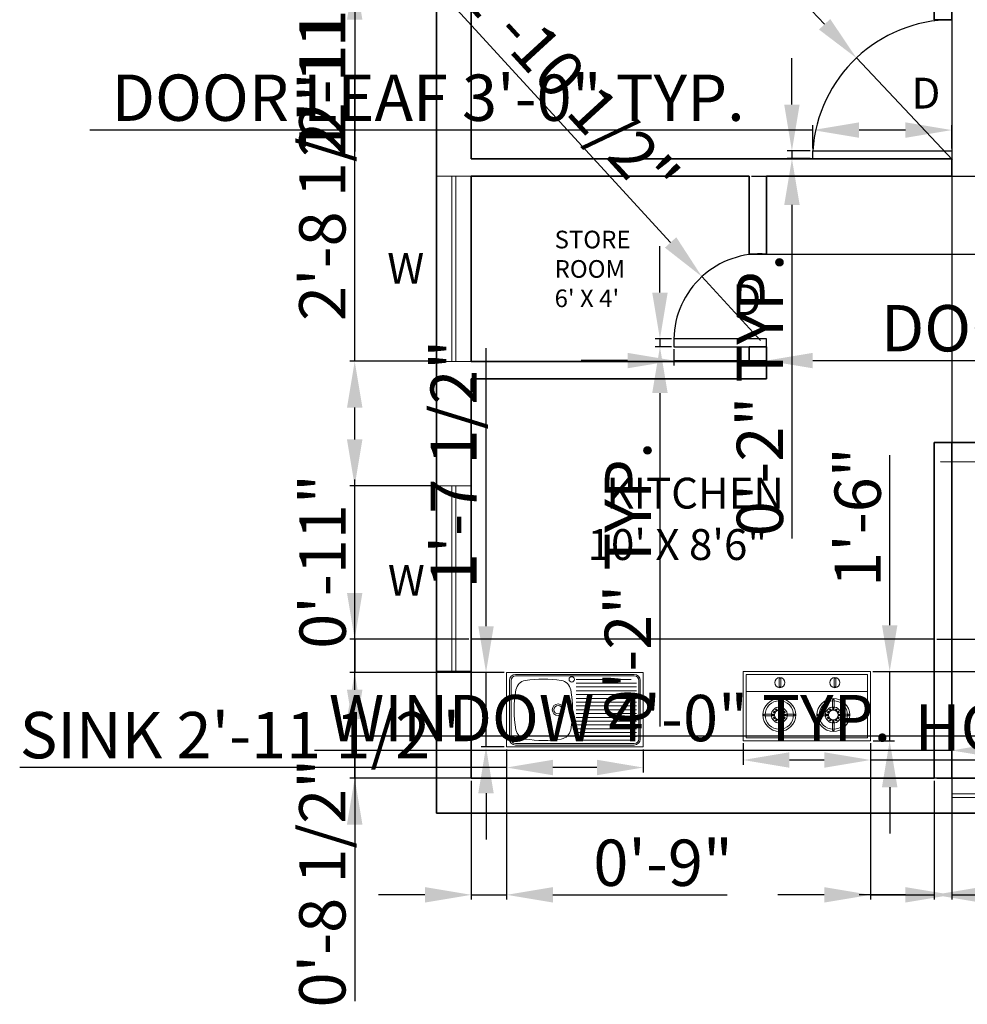
# Model space of a CAD drawing. Units: inches. Extents: x 2122 to 2726, y 1923 to 2370.
# Tile 1 of 6: x 2124 to 2370, y 1923 to 2178. Entities that reach past the tile are written whole.
import ezdxf

# ---------------------------------------------------------------- set-up
doc = ezdxf.new("R2010")
doc.units = ezdxf.units.IN
for name, color, linetype, lineweight in [('A-ANNO-DIMS', 2, 'Continuous', 18), ('A-ANNO-TEXT', 7, 'Continuous', 18), ('A-AREA-IDEN', 7, 'Continuous', 25), ('A-DOOR', 3, 'Continuous', 25), ('A-EQPM', 9, 'Continuous', 18), ('A-FLOR-CASE', 8, 'Continuous', 25), ('A-FLOR-FIXT', 9, 'Continuous', 18), ('A-GLAZ', 4, 'Continuous', 18), ('A-WALL', 7, 'Continuous', 35)]:
    doc.layers.add(name, color=color, linetype=linetype, lineweight=lineweight)
doc.styles.get("Standard").update_dxf_attribs({"font": 'arial.ttf'})
doc.dimstyles.new('ISO-25', dxfattribs={"dimtxt": 12, "dimasz": 12, "dimexe": 1.25, "dimexo": 0.625, "dimtad": 1, "dimlunit": 3, "dimtxsty": 'Standard', "dimcen": 2.5, "dimadec": 0, "dimazin": 0, "dimtfac": 1, "dimtmove": 0, "dimatfit": 3, "dimfxl": 1, "dimarcsym": 0})

# ---------------------------------------------------------------- blocks, each defined once
blk = doc.blocks.new('A$C06E242FC')
for p, q in [((0, 455.6), (0.5, 456.1)), ((0, 455.6), (0, 0.5)), ((838.9, 456.1), (0.5, 456.1)), ((838.9, 456.1), (839.4, 455.6)), ((839.4, 0.5), (839.4, 455.6)), ((20, 435.6), (20.5, 436.1)), ((20, 435.6), (20, 20.5)), ((818.9, 436.1), (20.5, 436.1)), ((237.3, 411.5), (237.3, 356.2)), ((248.9, 411.5), (237.3, 411.5)), ((248.9, 356.2), (248.9, 411.5)), ((599.3, 411.5), (610.9, 411.5)), ((599.3, 411.5), (599.3, 356.2)), ((610.9, 356.2), (610.9, 411.5)), ((819.4, 435.6), (818.9, 436.1)), ((819.4, 20.5), (819.4, 435.6)), ((20, 324.4), (819.4, 324.4)), ((237.3, 356.2), (248.9, 356.2)), ((599.3, 356.2), (610.9, 356.2)), ((232.7, 272.7), (232.7, 214)), ((244.9, 272.7), (232.7, 272.7)), ((244.9, 214), (244.9, 272.7)), ((588.1, 272.7), (588.1, 214)), ((600.3, 272.7), (588.1, 272.7)), ((600.3, 214), (600.3, 272.7)), ((232.7, 214), (244.9, 214)), ((588.1, 214), (600.3, 214)), ((136.3, 176), (136.3, 163.8)), ((194.9, 176), (136.3, 176)), ((136.3, 163.8), (194.9, 163.8)), ((194.9, 163.8), (194.9, 176)), ((282.9, 176.3), (282.9, 164.1)), ((341.6, 176.3), (282.9, 176.3)), ((282.9, 164.1), (341.6, 164.1)), ((341.6, 164.1), (341.6, 176.3)), ((550.3, 176), (491.7, 176)), ((491.7, 176), (491.7, 163.8)), ((491.7, 163.8), (550.3, 163.8)), ((550.3, 163.8), (550.3, 176)), ((638.3, 176.3), (638.3, 164.1)), ((697, 176.3), (638.3, 176.3)), ((638.3, 164.1), (697, 164.1)), ((697, 164.1), (697, 176.3)), ((245.2, 126.1), (233, 126.1)), ((233, 126.1), (233, 67.4)), ((233, 67.4), (245.2, 67.4)), ((245.2, 67.4), (245.2, 126.1)), ((600.6, 126.1), (588.3, 126.1)), ((588.3, 126.1), (588.3, 67.4)), ((588.3, 67.4), (600.6, 67.4)), ((600.6, 67.4), (600.6, 126.1)), ((0, 0.5), (0.5, 0)), ((20, 20.5), (20.5, 20)), ((20.5, 20), (818.9, 20)), ((818.9, 20), (819.4, 20.5)), ((838.9, 0), (839.4, 0.5)), ((0.5, 0), (838.9, 0))]:
    blk.add_line(p, q)
for centre, radius in [((242, 382.9), 33.3), ((604.1, 382.9), 33.3), ((238.9, 170.1), 108.3), ((238.9, 170.1), 93.3), ((594.3, 170.1), 108.3), ((594.3, 170.1), 93.3), ((238.9, 170.1), 52.6), ((238.9, 170.1), 32.6), ((219.5, 203.7), 4.84), ((238.9, 208.9), 4.84), ((258.4, 203.7), 4.84), ((594.3, 170.1), 52.6), ((594.3, 170.1), 32.6), ((574.9, 203.7), 4.84), ((594.3, 208.9), 4.84), ((613.7, 203.7), 4.84), ((200.1, 170.1), 4.84), ((205.3, 189.5), 4.84), ((205.3, 150.6), 4.84), ((219.5, 136.4), 4.84), ((238.9, 131.2), 4.84), ((258.4, 136.4), 4.84), ((272.6, 189.5), 4.84), ((272.6, 150.6), 4.84), ((277.8, 170.1), 4.84), ((555.5, 170.1), 4.84), ((560.7, 189.5), 4.84), ((560.7, 150.6), 4.84), ((574.9, 136.4), 4.84), ((594.3, 131.2), 4.84), ((613.7, 136.4), 4.84), ((628, 189.5), 4.84), ((628, 150.6), 4.84), ((633.2, 170.1), 4.84)]:
    blk.add_circle(centre, radius)
blk = doc.blocks.new('A$C0C3933DC')
for p, q in [((0, 490), (0, 0)), ((900, 490), (0, 490)), ((59.5, 477.5), (450, 477.5)), ((59.5, 467.5), (450, 467.5)), ((840.5, 477.5), (450, 477.5)), ((840.5, 467.5), (450, 467.5)), ((900, 0), (900, 490)), ((19.5, 52.5), (19.5, 437.5)), ((29.5, 52.5), (29.5, 437.5)), ((441, 420), (45, 420)), ((441, 395), (45, 395)), ((441, 445), (80.7, 445)), ((870.5, 52.5), (870.5, 437.5)), ((880.5, 52.5), (880.5, 437.5)), ((441, 370), (45, 370)), ((441, 345), (45, 345)), ((441, 320), (45, 320)), ((441, 295), (45, 295)), ((441, 270), (45, 270)), ((441, 245), (45, 245)), ((441, 220), (45, 220)), ((441, 195), (45, 195)), ((441, 170), (45, 170)), ((441, 145), (45, 145)), ((441, 120), (45, 120)), ((441, 95), (45, 95)), ((441, 70), (45, 70)), ((0, 0), (900, 0)), ((450, 22.5), (59.5, 22.5)), ((450, 12.5), (59.5, 12.5)), ((441, 45), (80.7, 45)), ((450, 22.5), (840.5, 22.5)), ((450, 12.5), (840.5, 12.5))]:
    blk.add_line(p, q)
for centre, radius in [((471, 445), 17.5), ((561, 245), 38), ((561, 245), 27.5)]:
    blk.add_circle(centre, radius)
for centre, radius, start, end in [((59.5, 437.5), 40, 90, 180), ((59.5, 437.5), 30, 90, 180), ((840.5, 437.5), 40, 0, 90), ((840.5, 437.5), 30, 0, 90), ((551.5, 363.5), 75, 99.07872, 169.88522), ((658, -303), 750, 80.92128, 99.07872), ((764.5, 363.5), 75, 10.11478, 80.92128), ((1216, 245), 750, 169.88522, 190.11478), ((100, 245), 750, 349.88522, 10.11478), ((551.5, 126.5), 75, 190.11478, 260.92128), ((764.5, 126.5), 75, 279.07872, 349.88522), ((59.5, 52.5), 40, 180, 270), ((59.5, 52.5), 30, 180, 270), ((658, 793), 750, 260.92128, 279.07872), ((840.5, 52.5), 30, 270, 0), ((840.5, 52.5), 40, 270, 0)]:
    blk.add_arc(centre, radius, start, end)
blk = doc.blocks.new('WIN-48IN')
for p, q in [((9, 48), (0, 48)), ((4, 0), (4, 48)), ((5, 0), (5, 48)), ((9, 0), (0, 0))]:
    blk.add_line(p, q)
blk = doc.blocks.new('DOOR-LEAF-36IN')
for p, q in [((0, 2), (36, 2)), ((0, 0), (0, 2)), ((36, 0), (0, 0)), ((36, 2), (36, 0))]:
    blk.add_line(p, q)
blk = doc.blocks.new('DOOR-LEAF-24IN')
for p, q in [((2, 24), (0, 24)), ((0, 24), (0, 0)), ((2, 0), (2, 24)), ((0, 0), (2, 0))]:
    blk.add_line(p, q)
blk = doc.blocks.new('*D18')
at = {"layer": 'A-ANNO-DIMS', "color": 0, "lineweight": -2, "transparency": 16777216}
for p, q in [((2366.01, 1982.36), (2366.01, 1990.19)), ((2414.01, 1982.36), (2414.01, 1990.19)), ((2366.01, 1988.94), (2200.91, 1988.94)), ((2402.01, 1988.94), (2378.01, 1988.94))]:
    blk.add_line(p, q, dxfattribs=at)
at = {"layer": 'A-ANNO-DIMS', "color": 0, "transparency": 16777216}
for points in [[(2378.01, 1990.94), (2378.01, 1986.94), (2366.01, 1988.94)], [(2402.01, 1990.94), (2402.01, 1986.94), (2414.01, 1988.94)]]:
    blk.add_solid(points, dxfattribs=at)
at = {"layer": 'Defpoints', "color": 0, "transparency": 16777216}
for p in [(2366.01, 1988.94), (2366.01, 1981.74), (2414.01, 1981.74)]:
    blk.add_point(p, dxfattribs=at)
at = {"layer": 'A-ANNO-DIMS', "color": 0, "transparency": 16777216, "insert": (2277.46, 1995.77), "char_height": 12, "attachment_point": 5}
blk.add_mtext('WINDOW 4\'-0" TYP.', dxfattribs=at)
blk = doc.blocks.new('*D22')
at = {"layer": 'A-ANNO-DIMS', "color": 0, "lineweight": -2, "transparency": 16777216}
for p, q in [((2330.01, 2144.86), (2330.01, 2150.89)), ((2366.01, 2144.86), (2366.01, 2150.89)), ((2330.01, 2149.64), (2142.68, 2149.64)), ((2354.01, 2149.64), (2342.01, 2149.64))]:
    blk.add_line(p, q, dxfattribs=at)
at = {"layer": 'A-ANNO-DIMS', "color": 0, "transparency": 16777216}
for points in [[(2342.01, 2151.64), (2342.01, 2147.64), (2330.01, 2149.64)], [(2354.01, 2151.64), (2354.01, 2147.64), (2366.01, 2149.64)]]:
    blk.add_solid(points, dxfattribs=at)
at = {"layer": 'Defpoints', "color": 0, "transparency": 16777216}
for p in [(2330.01, 2149.64), (2330.01, 2144.24), (2366.01, 2144.24)]:
    blk.add_point(p, dxfattribs=at)
at = {"layer": 'A-ANNO-DIMS', "color": 0, "transparency": 16777216, "insert": (2230.34, 2156.47), "char_height": 12, "attachment_point": 5}
blk.add_mtext('DOOR LEAF 3\'-0" TYP.', dxfattribs=at)
blk = doc.blocks.new('*D23')
at = {"layer": 'A-ANNO-DIMS', "color": 0, "lineweight": -2, "transparency": 16777216}
for p, q in [((2324.61, 2156.24), (2324.61, 2168.24)), ((2329.38, 2144.24), (2323.36, 2144.24)), ((2324.61, 2144.24), (2324.61, 2142.24)), ((2329.38, 2142.24), (2323.36, 2142.24)), ((2324.61, 2130.24), (2324.61, 2043.84))]:
    blk.add_line(p, q, dxfattribs=at)
at = {"layer": 'A-ANNO-DIMS', "color": 0, "transparency": 16777216}
for points in [[(2322.61, 2156.24), (2326.61, 2156.24), (2324.61, 2144.24)], [(2322.61, 2130.24), (2326.61, 2130.24), (2324.61, 2142.24)]]:
    blk.add_solid(points, dxfattribs=at)
at = {"layer": 'Defpoints', "color": 0, "transparency": 16777216}
for p in [(2330.01, 2144.24), (2324.61, 2142.24), (2330.01, 2142.24)]:
    blk.add_point(p, dxfattribs=at)
at = {"layer": 'A-ANNO-DIMS', "color": 0, "transparency": 16777216, "insert": (2317.86, 2081.04), "char_height": 12, "attachment_point": 5, "rotation": 90}
blk.add_mtext('0\'-2" TYP.', dxfattribs=at)
blk = doc.blocks.new('*D24')
at = {"layer": 'A-ANNO-DIMS', "color": 0, "lineweight": -2, "transparency": 16777216}
for p, q in [((2294.01, 2092.91), (2294.01, 2088.68)), ((2318.01, 2092.91), (2318.01, 2088.68)), ((2282.01, 2089.93), (2270.01, 2089.93)), ((2294.01, 2089.93), (2318.01, 2089.93)), ((2330.01, 2089.93), (2517.34, 2089.93))]:
    blk.add_line(p, q, dxfattribs=at)
at = {"layer": 'A-ANNO-DIMS', "color": 0, "transparency": 16777216}
for points in [[(2282.01, 2091.93), (2282.01, 2087.93), (2294.01, 2089.93)], [(2330.01, 2091.93), (2330.01, 2087.93), (2318.01, 2089.93)]]:
    blk.add_solid(points, dxfattribs=at)
at = {"layer": 'Defpoints', "color": 0, "transparency": 16777216}
for p in [(2294.01, 2093.53), (2318.01, 2093.53), (2318.01, 2089.93)]:
    blk.add_point(p, dxfattribs=at)
at = {"layer": 'A-ANNO-DIMS', "color": 0, "transparency": 16777216, "insert": (2429.67, 2096.76), "char_height": 12, "attachment_point": 5}
blk.add_mtext('DOOR LEAF 2\'-0" TYP.', dxfattribs=at)
blk = doc.blocks.new('*D25')
at = {"layer": 'A-ANNO-DIMS', "color": 0, "lineweight": -2, "transparency": 16777216}
for p, q in [((2290.41, 2107.53), (2290.41, 2119.53)), ((2293.38, 2095.53), (2289.16, 2095.53)), ((2290.41, 2095.53), (2290.41, 2093.53)), ((2293.38, 2093.53), (2289.16, 2093.53)), ((2290.41, 2081.53), (2290.41, 1995.13))]:
    blk.add_line(p, q, dxfattribs=at)
at = {"layer": 'A-ANNO-DIMS', "color": 0, "transparency": 16777216}
for points in [[(2288.41, 2107.53), (2292.41, 2107.53), (2290.41, 2095.53)], [(2288.41, 2081.53), (2292.41, 2081.53), (2290.41, 2093.53)]]:
    blk.add_solid(points, dxfattribs=at)
at = {"layer": 'Defpoints', "color": 0, "transparency": 16777216}
for p in [(2294.01, 2095.53), (2290.41, 2093.53), (2294.01, 2093.53)]:
    blk.add_point(p, dxfattribs=at)
at = {"layer": 'A-ANNO-DIMS', "color": 0, "transparency": 16777216, "insert": (2283.66, 2032.33), "char_height": 12, "attachment_point": 5, "rotation": 90}
blk.add_mtext('0\'-2" TYP.', dxfattribs=at)
blk = doc.blocks.new('*D30')
at = {"layer": 'A-ANNO-DIMS', "color": 0, "lineweight": -2, "transparency": 16777216}
for p, q in [((2311.94, 1990.8), (2311.94, 1985.22)), ((2344.99, 1990.8), (2344.99, 1985.22)), ((2323.94, 1986.47), (2332.99, 1986.47)), ((2344.99, 1986.47), (2430.48, 1986.47))]:
    blk.add_line(p, q, dxfattribs=at)
at = {"layer": 'A-ANNO-DIMS', "color": 0, "transparency": 16777216}
for points in [[(2323.94, 1988.47), (2323.94, 1984.47), (2311.94, 1986.47)], [(2332.99, 1988.47), (2332.99, 1984.47), (2344.99, 1986.47)]]:
    blk.add_solid(points, dxfattribs=at)
at = {"layer": 'Defpoints', "color": 0, "transparency": 16777216}
for p in [(2311.94, 1991.43), (2344.99, 1991.43), (2344.99, 1986.47)]:
    blk.add_point(p, dxfattribs=at)
at = {"layer": 'A-ANNO-DIMS', "color": 0, "transparency": 16777216, "insert": (2393.73, 1993.3), "char_height": 12, "attachment_point": 5}
blk.add_mtext('HOB 2\'-9"', dxfattribs=at)
blk = doc.blocks.new('*D31')
at = {"layer": 'A-ANNO-DIMS', "color": 0, "lineweight": -2, "transparency": 16777216}
for p, q in [((2349.95, 2021.39), (2349.95, 2065.4)), ((2345.62, 2009.39), (2351.2, 2009.39)), ((2349.95, 1991.43), (2349.95, 2009.39)), ((2345.62, 1991.43), (2351.2, 1991.43)), ((2349.95, 1979.43), (2349.95, 1967.43))]:
    blk.add_line(p, q, dxfattribs=at)
at = {"layer": 'A-ANNO-DIMS', "color": 0, "transparency": 16777216}
for points in [[(2347.95, 2021.39), (2351.95, 2021.39), (2349.95, 2009.39)], [(2347.95, 1979.43), (2351.95, 1979.43), (2349.95, 1991.43)]]:
    blk.add_solid(points, dxfattribs=at)
at = {"layer": 'Defpoints', "color": 0, "transparency": 16777216}
for p in [(2344.99, 2009.39), (2349.95, 2009.39), (2344.99, 1991.43)]:
    blk.add_point(p, dxfattribs=at)
at = {"layer": 'A-ANNO-DIMS', "color": 0, "transparency": 16777216, "insert": (2343.2, 2049.39), "char_height": 12, "attachment_point": 5, "rotation": 90}
blk.add_mtext('1\'-6"', dxfattribs=at)
blk = doc.blocks.new('*D32')
at = {"layer": 'A-ANNO-DIMS', "color": 0, "lineweight": -2, "transparency": 16777216}
for p, q in [((2250.66, 1989.21), (2250.66, 1983.27)), ((2286.09, 1989.21), (2286.09, 1983.27)), ((2250.66, 1984.52), (2124.5, 1984.52)), ((2274.09, 1984.52), (2262.66, 1984.52))]:
    blk.add_line(p, q, dxfattribs=at)
at = {"layer": 'A-ANNO-DIMS', "color": 0, "transparency": 16777216}
for points in [[(2262.66, 1986.52), (2262.66, 1982.52), (2250.66, 1984.52)], [(2274.09, 1986.52), (2274.09, 1982.52), (2286.09, 1984.52)]]:
    blk.add_solid(points, dxfattribs=at)
at = {"layer": 'Defpoints', "color": 0, "transparency": 16777216}
for p in [(2250.66, 1989.84), (2286.09, 1989.84), (2250.66, 1984.52)]:
    blk.add_point(p, dxfattribs=at)
at = {"layer": 'A-ANNO-DIMS', "color": 0, "transparency": 16777216, "insert": (2181.58, 1991.35), "char_height": 12, "attachment_point": 5}
blk.add_mtext('SINK 2\'-11 1/2"', dxfattribs=at)
blk = doc.blocks.new('*D33')
at = {"layer": 'A-ANNO-DIMS', "color": 0, "lineweight": -2, "transparency": 16777216}
for p, q in [((2245.34, 2021.13), (2245.34, 2093.11)), ((2250.03, 2009.13), (2244.09, 2009.13)), ((2245.34, 1989.84), (2245.34, 2009.13)), ((2250.03, 1989.84), (2244.09, 1989.84)), ((2245.34, 1977.84), (2245.34, 1965.84))]:
    blk.add_line(p, q, dxfattribs=at)
at = {"layer": 'A-ANNO-DIMS', "color": 0, "transparency": 16777216}
for points in [[(2243.34, 2021.13), (2247.34, 2021.13), (2245.34, 2009.13)], [(2243.34, 1977.84), (2247.34, 1977.84), (2245.34, 1989.84)]]:
    blk.add_solid(points, dxfattribs=at)
at = {"layer": 'Defpoints', "color": 0, "transparency": 16777216}
for p in [(2245.34, 2009.13), (2250.66, 2009.13), (2250.66, 1989.84)]:
    blk.add_point(p, dxfattribs=at)
at = {"layer": 'A-ANNO-DIMS', "color": 0, "transparency": 16777216, "insert": (2238.51, 2063.12), "char_height": 12, "attachment_point": 5, "rotation": 90}
blk.add_mtext('1\'-7 1/2"', dxfattribs=at)
blk = doc.blocks.new('*D40')
at = {"layer": 'A-ANNO-DIMS', "color": 0, "lineweight": -2, "transparency": 16777216}
for p, q in [((2362.13, 2017.74), (2622.46, 2017.74)), ((2621.21, 1993.74), (2621.21, 2005.74)), ((2362.13, 1981.74), (2622.46, 1981.74))]:
    blk.add_line(p, q, dxfattribs=at)
at = {"layer": 'A-ANNO-DIMS', "color": 0, "transparency": 16777216}
for points in [[(2619.21, 2005.74), (2623.21, 2005.74), (2621.21, 2017.74)], [(2619.21, 1993.74), (2623.21, 1993.74), (2621.21, 1981.74)]]:
    blk.add_solid(points, dxfattribs=at)
at = {"layer": 'Defpoints', "color": 0, "transparency": 16777216}
for p in [(2361.51, 2017.74), (2621.21, 2017.74), (2361.51, 1981.74)]:
    blk.add_point(p, dxfattribs=at)
at = {"layer": 'A-ANNO-DIMS', "color": 0, "transparency": 16777216, "insert": (2614.45, 1999.74), "char_height": 12, "attachment_point": 5, "rotation": 90}
blk.add_mtext('3\'-0"', dxfattribs=at)
blk = doc.blocks.new('*D45')
at = {"layer": 'A-ANNO-DIMS', "color": 0, "lineweight": -2, "transparency": 16777216}
for p, q in [((2211.31, 2089.74), (2211.31, 2163.05)), ((2231.88, 2089.74), (2210.06, 2089.74)), ((2211.31, 2069.49), (2211.31, 2077.74)), ((2231.88, 2057.49), (2210.06, 2057.49))]:
    blk.add_line(p, q, dxfattribs=at)
at = {"layer": 'A-ANNO-DIMS', "color": 0, "transparency": 16777216}
for points in [[(2209.31, 2077.74), (2213.31, 2077.74), (2211.31, 2089.74)], [(2209.31, 2069.49), (2213.31, 2069.49), (2211.31, 2057.49)]]:
    blk.add_solid(points, dxfattribs=at)
at = {"layer": 'Defpoints', "color": 0, "transparency": 16777216}
for p in [(2211.31, 2089.74), (2232.51, 2089.74), (2232.51, 2057.49)]:
    blk.add_point(p, dxfattribs=at)
at = {"layer": 'A-ANNO-DIMS', "color": 0, "transparency": 16777216, "insert": (2204.48, 2132.39), "char_height": 12, "attachment_point": 5, "rotation": 90}
blk.add_mtext('2\'-8 1/2"', dxfattribs=at)
blk = doc.blocks.new('*D50')
at = {"layer": 'A-ANNO-DIMS', "color": 0, "lineweight": -2, "transparency": 16777216}
for p, q in [((2366.01, 2189.61), (2366.01, 1950.29)), ((2385.88, 2189.61), (2385.88, 1950.29)), ((2354.01, 1951.54), (2342.01, 1951.54)), ((2366.01, 1951.54), (2385.88, 1951.54)), ((2397.88, 1951.54), (2441.9, 1951.54))]:
    blk.add_line(p, q, dxfattribs=at)
at = {"layer": 'A-ANNO-DIMS', "color": 0, "transparency": 16777216}
for points in [[(2354.01, 1953.54), (2354.01, 1949.54), (2366.01, 1951.54)], [(2397.88, 1953.54), (2397.88, 1949.54), (2385.88, 1951.54)]]:
    blk.add_solid(points, dxfattribs=at)
at = {"layer": 'Defpoints', "color": 0, "transparency": 16777216}
for p in [(2366.01, 2190.24), (2385.88, 2190.24), (2385.88, 1951.54)]:
    blk.add_point(p, dxfattribs=at)
at = {"layer": 'A-ANNO-DIMS', "color": 0, "transparency": 16777216, "insert": (2425.89, 1958.29), "char_height": 12, "attachment_point": 5}
blk.add_mtext('1\'-8"', dxfattribs=at)
blk = doc.blocks.new('*D51')
at = {"layer": 'A-ANNO-DIMS', "color": 0, "lineweight": -2, "transparency": 16777216}
for p, q in [((2211.31, 2209.57), (2211.31, 2282.68)), ((2465.88, 2197.57), (2210.06, 2197.57)), ((2211.31, 2190.24), (2211.31, 2197.57)), ((2465.88, 2190.24), (2210.06, 2190.24)), ((2211.31, 2178.24), (2211.31, 2166.24))]:
    blk.add_line(p, q, dxfattribs=at)
at = {"layer": 'A-ANNO-DIMS', "color": 0, "transparency": 16777216}
for points in [[(2209.31, 2209.57), (2213.31, 2209.57), (2211.31, 2197.57)], [(2209.31, 2178.24), (2213.31, 2178.24), (2211.31, 2190.24)]]:
    blk.add_solid(points, dxfattribs=at)
at = {"layer": 'Defpoints', "color": 0, "transparency": 16777216}
for p in [(2211.31, 2197.57), (2466.51, 2197.57), (2466.51, 2190.24)]:
    blk.add_point(p, dxfattribs=at)
at = {"layer": 'A-ANNO-DIMS', "color": 0, "transparency": 16777216, "insert": (2204.48, 2252.12), "char_height": 12, "attachment_point": 5, "rotation": 90}
blk.add_mtext('0\'-7 1/2"', dxfattribs=at)
blk = doc.blocks.new('*D52')
at = {"layer": 'A-ANNO-DIMS', "color": 0, "lineweight": -2, "transparency": 16777216}
for p, q in [((2621.21, 2149.74), (2621.21, 2161.74)), ((2314.13, 2137.74), (2622.46, 2137.74)), ((2621.21, 2137.74), (2621.21, 2117.53)), ((2314.13, 2117.53), (2622.46, 2117.53)), ((2621.21, 2105.53), (2621.21, 2061.51))]:
    blk.add_line(p, q, dxfattribs=at)
at = {"layer": 'A-ANNO-DIMS', "color": 0, "transparency": 16777216}
for points in [[(2619.21, 2149.74), (2623.21, 2149.74), (2621.21, 2137.74)], [(2619.21, 2105.53), (2623.21, 2105.53), (2621.21, 2117.53)]]:
    blk.add_solid(points, dxfattribs=at)
at = {"layer": 'Defpoints', "color": 0, "transparency": 16777216}
for p in [(2313.51, 2137.74), (2313.51, 2117.53), (2621.21, 2117.53)]:
    blk.add_point(p, dxfattribs=at)
at = {"layer": 'A-ANNO-DIMS', "color": 0, "transparency": 16777216, "insert": (2614.46, 2077.52), "char_height": 12, "attachment_point": 5, "rotation": 90}
blk.add_mtext('1\'-8"', dxfattribs=at)
blk = doc.blocks.new('*D53')
at = {"layer": 'A-ANNO-DIMS', "color": 0, "lineweight": -2, "transparency": 16777216}
for p, q in [((2250.66, 1989.21), (2250.66, 1950.29)), ((2241.51, 1981.11), (2241.51, 1950.29)), ((2229.51, 1951.54), (2217.51, 1951.54)), ((2241.51, 1951.54), (2250.66, 1951.54)), ((2262.66, 1951.54), (2307.81, 1951.54))]:
    blk.add_line(p, q, dxfattribs=at)
at = {"layer": 'A-ANNO-DIMS', "color": 0, "transparency": 16777216}
for points in [[(2229.51, 1953.54), (2229.51, 1949.54), (2241.51, 1951.54)], [(2262.66, 1953.54), (2262.66, 1949.54), (2250.66, 1951.54)]]:
    blk.add_solid(points, dxfattribs=at)
at = {"layer": 'Defpoints', "color": 0, "transparency": 16777216}
for p in [(2250.66, 1989.84), (2241.51, 1981.74), (2250.66, 1951.54)]:
    blk.add_point(p, dxfattribs=at)
at = {"layer": 'A-ANNO-DIMS', "color": 0, "transparency": 16777216, "insert": (2291.23, 1958.29), "char_height": 12, "attachment_point": 5}
blk.add_mtext('0\'-9"', dxfattribs=at)
blk = doc.blocks.new('*D54')
at = {"layer": 'A-ANNO-DIMS', "color": 0, "lineweight": -2, "transparency": 16777216}
for p, q in [((2211.31, 2029.74), (2211.31, 2041.74)), ((2240.88, 2017.74), (2210.06, 2017.74)), ((2211.31, 2017.74), (2211.31, 2009.13)), ((2250.03, 2009.13), (2210.06, 2009.13)), ((2211.31, 1997.13), (2211.31, 1924.02))]:
    blk.add_line(p, q, dxfattribs=at)
at = {"layer": 'A-ANNO-DIMS', "color": 0, "transparency": 16777216}
for points in [[(2209.31, 2029.74), (2213.31, 2029.74), (2211.31, 2017.74)], [(2209.31, 1997.13), (2213.31, 1997.13), (2211.31, 2009.13)]]:
    blk.add_solid(points, dxfattribs=at)
at = {"layer": 'Defpoints', "color": 0, "transparency": 16777216}
for p in [(2241.51, 2017.74), (2211.31, 2009.13), (2250.66, 2009.13)]:
    blk.add_point(p, dxfattribs=at)
at = {"layer": 'A-ANNO-DIMS', "color": 0, "transparency": 16777216, "insert": (2204.48, 1954.57), "char_height": 12, "attachment_point": 5, "rotation": 90}
blk.add_mtext('0\'-8 1/2"', dxfattribs=at)
blk = doc.blocks.new('*D55')
at = {"layer": 'A-ANNO-DIMS', "color": 0, "lineweight": -2, "transparency": 16777216}
for p, q in [((2344.97, 1990.8), (2344.97, 1950.29)), ((2361.51, 1981.11), (2361.51, 1950.29)), ((2332.97, 1951.54), (2320.97, 1951.54)), ((2344.97, 1951.54), (2361.51, 1951.54)), ((2373.51, 1951.54), (2445.49, 1951.54))]:
    blk.add_line(p, q, dxfattribs=at)
at = {"layer": 'A-ANNO-DIMS', "color": 0, "transparency": 16777216}
for points in [[(2332.97, 1953.54), (2332.97, 1949.54), (2344.97, 1951.54)], [(2373.51, 1953.54), (2373.51, 1949.54), (2361.51, 1951.54)]]:
    blk.add_solid(points, dxfattribs=at)
at = {"layer": 'Defpoints', "color": 0, "transparency": 16777216}
for p in [(2344.97, 1991.43), (2361.51, 1981.74), (2361.51, 1951.54)]:
    blk.add_point(p, dxfattribs=at)
at = {"layer": 'A-ANNO-DIMS', "color": 0, "transparency": 16777216, "insert": (2415.5, 1958.37), "char_height": 12, "attachment_point": 5}
blk.add_mtext('1\'-4 1/2"', dxfattribs=at)
blk = doc.blocks.new('*D56')
at = {"layer": 'A-ANNO-DIMS', "color": 0, "lineweight": -2, "transparency": 16777216}
for p, q in [((2621.21, 2029.74), (2621.21, 2102.85)), ((2362.13, 2017.74), (2622.46, 2017.74)), ((2621.21, 2009.39), (2621.21, 2017.74)), ((2345.6, 2009.39), (2622.46, 2009.39)), ((2621.21, 1997.39), (2621.21, 1985.39))]:
    blk.add_line(p, q, dxfattribs=at)
at = {"layer": 'A-ANNO-DIMS', "color": 0, "transparency": 16777216}
for points in [[(2619.21, 2029.74), (2623.21, 2029.74), (2621.21, 2017.74)], [(2619.21, 1997.39), (2623.21, 1997.39), (2621.21, 2009.39)]]:
    blk.add_solid(points, dxfattribs=at)
at = {"layer": 'Defpoints', "color": 0, "transparency": 16777216}
for p in [(2361.51, 2017.74), (2621.21, 2017.74), (2344.97, 2009.39)]:
    blk.add_point(p, dxfattribs=at)
at = {"layer": 'A-ANNO-DIMS', "color": 0, "transparency": 16777216, "insert": (2614.38, 2072.29), "char_height": 12, "attachment_point": 5, "rotation": 90}
blk.add_mtext('0\'-8 1/2"', dxfattribs=at)
blk = doc.blocks.new('*D59')
at = {"layer": 'A-ANNO-DIMS', "color": 0, "lineweight": -2, "transparency": 16777216}
for p, q in [((2211.31, 2004.66), (2211.31, 2059.13)), ((2481.63, 1992.66), (2210.06, 1992.66)), ((2211.31, 1981.74), (2211.31, 1992.66)), ((2470.38, 1981.74), (2210.06, 1981.74)), ((2211.31, 1969.74), (2211.31, 1957.74))]:
    blk.add_line(p, q, dxfattribs=at)
at = {"layer": 'A-ANNO-DIMS', "color": 0, "transparency": 16777216}
for points in [[(2209.31, 2004.66), (2213.31, 2004.66), (2211.31, 1992.66)], [(2209.31, 1969.74), (2213.31, 1969.74), (2211.31, 1981.74)]]:
    blk.add_solid(points, dxfattribs=at)
at = {"layer": 'Defpoints', "color": 0, "transparency": 16777216}
for p in [(2211.31, 1992.66), (2482.26, 1992.66), (2471.01, 1981.74)]:
    blk.add_point(p, dxfattribs=at)
at = {"layer": 'A-ANNO-DIMS', "color": 0, "transparency": 16777216, "insert": (2204.56, 2037.89), "char_height": 12, "attachment_point": 5, "rotation": 90}
blk.add_mtext('0\'-11"', dxfattribs=at)
blk = doc.blocks.new('*D61')
at = {"layer": 'A-ANNO-DIMS', "color": 0, "lineweight": -2, "transparency": 16777216}
for p, q in [((2240.88, 2262.24), (2210.06, 2262.24)), ((2211.31, 2250.24), (2211.31, 2238.75)), ((2246.26, 2226.75), (2210.06, 2226.75)), ((2211.31, 2226.75), (2211.31, 2144.11))]:
    blk.add_line(p, q, dxfattribs=at)
at = {"layer": 'A-ANNO-DIMS', "color": 0, "transparency": 16777216}
for points in [[(2209.31, 2250.24), (2213.31, 2250.24), (2211.31, 2262.24)], [(2209.31, 2238.75), (2213.31, 2238.75), (2211.31, 2226.75)]]:
    blk.add_solid(points, dxfattribs=at)
at = {"layer": 'Defpoints', "color": 0, "transparency": 16777216}
for p in [(2241.51, 2262.24), (2211.31, 2226.75), (2246.89, 2226.75)]:
    blk.add_point(p, dxfattribs=at)
at = {"layer": 'A-ANNO-DIMS', "color": 0, "transparency": 16777216, "insert": (2204.48, 2179.43), "char_height": 12, "attachment_point": 5, "rotation": 90}
blk.add_mtext('2\'-11 1/2"', dxfattribs=at)
blk = doc.blocks.new('*D65')
at = {"layer": 'A-ANNO-DIMS', "color": 0, "lineweight": -2, "transparency": 16777216}
for p, q in [((2211.31, 2274.24), (2211.31, 2286.24)), ((2413.38, 2262.24), (2210.06, 2262.24)), ((2211.31, 2262.24), (2211.31, 2238.81)), ((2409.54, 2238.81), (2210.06, 2238.81)), ((2211.31, 2226.81), (2211.31, 2145.5))]:
    blk.add_line(p, q, dxfattribs=at)
at = {"layer": 'A-ANNO-DIMS', "color": 0, "transparency": 16777216}
for points in [[(2209.31, 2274.24), (2213.31, 2274.24), (2211.31, 2262.24)], [(2209.31, 2226.81), (2213.31, 2226.81), (2211.31, 2238.81)]]:
    blk.add_solid(points, dxfattribs=at)
at = {"layer": 'Defpoints', "color": 0, "transparency": 16777216}
for p in [(2414.01, 2262.24), (2211.31, 2238.81), (2410.17, 2238.81)]:
    blk.add_point(p, dxfattribs=at)
at = {"layer": 'A-ANNO-DIMS', "color": 0, "transparency": 16777216, "insert": (2204.48, 2180.16), "char_height": 12, "attachment_point": 5, "rotation": 90}
blk.add_mtext('1\'-11 1/2"', dxfattribs=at)
blk = doc.blocks.new('*D70')
at = {"layer": 'A-ANNO-DIMS', "color": 0, "lineweight": -2, "transparency": 16777216}
for p, q in [((2274.99, 2238.55), (2333.07, 2177.05)), ((2366.24, 2141.93), (2341.31, 2168.33))]:
    blk.add_line(p, q, dxfattribs=at)
at = {"layer": 'A-ANNO-DIMS', "color": 0, "transparency": 16777216}
blk.add_solid([(2334.53, 2178.42), (2331.62, 2175.68), (2341.31, 2168.33)], dxfattribs=at)
at = {"layer": 'Defpoints', "color": 0, "transparency": 16777216}
for p in [(2341.31, 2168.33), (2366.24, 2141.93)]:
    blk.add_point(p, dxfattribs=at)
at = {"layer": 'A-ANNO-DIMS', "color": 0, "transparency": 16777216, "insert": (2304.88, 2216.85), "char_height": 12, "attachment_point": 5, "rotation": 313.3629}
blk.add_mtext('R3\'-0 1/2"', dxfattribs=at)
blk = doc.blocks.new('*D73')
at = {"layer": 'A-ANNO-DIMS', "color": 0, "lineweight": -2, "transparency": 16777216}
for p, q in [((2229.71, 2189.76), (2293.17, 2120.53)), ((2316.45, 2095.14), (2301.28, 2111.68))]:
    blk.add_line(p, q, dxfattribs=at)
at = {"layer": 'A-ANNO-DIMS', "color": 0, "transparency": 16777216}
blk.add_solid([(2294.65, 2121.88), (2291.7, 2119.18), (2301.28, 2111.68)], dxfattribs=at)
at = {"layer": 'Defpoints', "color": 0, "transparency": 16777216}
for p in [(2301.28, 2111.68), (2316.45, 2095.14)]:
    blk.add_point(p, dxfattribs=at)
at = {"layer": 'A-ANNO-DIMS', "color": 0, "transparency": 16777216, "insert": (2262.42, 2164.19), "char_height": 12, "attachment_point": 5, "rotation": 312.5099}
blk.add_mtext('R1\'-10 1/2"', dxfattribs=at)
blk = doc.blocks.new('*D76')
at = {"layer": 'A-ANNO-DIMS', "color": 0, "lineweight": -2, "transparency": 16777216}
for p, q in [((2375.12, 2063.64), (2363.12, 2063.73)), ((2387.12, 2063.55), (2394.08, 2063.5)), ((2464.28, 2062.99), (2406.08, 2063.41))]:
    blk.add_line(p, q, dxfattribs=at)
at = {"layer": 'A-ANNO-DIMS', "color": 0, "transparency": 16777216}
for points in [[(2375.13, 2065.64), (2375.1, 2061.64), (2387.12, 2063.55)], [(2406.09, 2065.41), (2406.07, 2061.41), (2394.08, 2063.5)]]:
    blk.add_solid(points, dxfattribs=at)
at = {"layer": 'Defpoints', "color": 0, "transparency": 16777216}
for p in [(2387.12, 2063.55), (2394.08, 2063.5)]:
    blk.add_point(p, dxfattribs=at)
at = {"layer": 'A-ANNO-DIMS', "color": 0, "transparency": 16777216, "insert": (2441.23, 2070.24), "char_height": 12, "attachment_point": 5, "rotation": 359.5814}
blk.add_mtext('∅0\'-7"', dxfattribs=at)

msp = doc.modelspace()

# ---------------------------------------------------------------- linework, layer by layer
at = {"layer": 'A-DOOR'}
for centre, radius, start, end in [((2366.243, 2141.928), 36.309, 90.37146, 176.35538), ((2316.451, 2095.138), 22.447, 86.02325, 178.99765)]:
    msp.add_arc(centre, radius, start, end, dxfattribs=at)
at = {"layer": 'A-FLOR-CASE'}
msp.add_line((2361.508, 2017.736), (2241.508, 2017.736), dxfattribs=at)
at = {"layer": 'A-WALL'}
for p, q in [((2232.508, 2271.236), (2232.508, 2142.236)), ((2241.508, 2262.236), (2241.508, 2142.236)), ((2361.508, 2178.236), (2361.508, 2262.236)), ((2366.008, 2178.236), (2366.008, 2185.736)), ((2361.508, 2178.236), (2366.008, 2178.236)), ((2232.508, 2142.236), (2232.508, 1972.736)), ((2241.508, 2142.236), (2361.508, 2142.236)), ((2361.508, 2142.236), (2366.008, 2142.236)), ((2366.008, 2137.736), (2366.008, 2142.236)), ((2241.508, 2137.736), (2313.508, 2137.736)), ((2241.508, 2137.736), (2241.508, 2089.736)), ((2313.508, 2137.736), (2313.508, 2117.531)), ((2318.008, 2137.736), (2318.008, 2117.531)), ((2318.008, 2137.736), (2366.008, 2137.736)), ((2313.508, 2117.531), (2318.008, 2117.531)), ((2313.508, 2093.531), (2318.008, 2093.531)), ((2313.508, 2093.531), (2313.508, 2089.736)), ((2318.008, 2093.531), (2318.008, 2089.736)), ((2241.508, 2089.736), (2313.508, 2089.736)), ((2318.008, 2089.736), (2318.008, 2085.236)), ((2241.508, 2085.236), (2318.008, 2085.236)), ((2241.508, 2085.236), (2241.508, 1981.736)), ((2361.508, 2068.736), (2361.508, 1981.736)), ((2418.508, 2068.736), (2361.508, 2068.736)), ((2366.008, 2068.736), (2366.008, 1981.736)), ((2361.508, 1981.736), (2241.508, 1981.736)), ((2414.008, 1981.736), (2366.008, 1981.736)), ((2418.508, 1972.736), (2232.508, 1972.736))]:
    msp.add_line(p, q, dxfattribs=at)

# ---------------------------------------------------------------- block references
at = {"layer": 'A-DOOR'}
for name, p, rotation in [('DOOR-LEAF-36IN', (2366.007, 2144.236), 180), ('DOOR-LEAF-24IN', (2294.008, 2095.53), 270)]:
    msp.add_blockref(name, p, dxfattribs=dict(at, rotation=rotation))
at = {"layer": 'A-EQPM', "xscale": 0.0393700787401575, "yscale": 0.0393700787401575, "zscale": 0.0393700787401575}
msp.add_blockref('A$C06E242FC', (2311.944, 1991.428), dxfattribs=at)
at = {"layer": 'A-FLOR-FIXT', "xscale": -0.0393700787401575, "yscale": 0.0393700787401575, "zscale": 0.0393700787401575}
msp.add_blockref('A$C0C3933DC', (2286.091, 1989.839), dxfattribs=at)
at = {"layer": 'A-GLAZ'}
for p, rotation in [((2241.507, 2137.736), 180), ((2414.008, 1972.736), 89.99999999999747)]:
    msp.add_blockref('WIN-48IN', p, dxfattribs=dict(at, rotation=rotation))
msp.add_blockref('WIN-48IN', (2232.508, 2009.486), dxfattribs=at)

# ---------------------------------------------------------------- texts
at = {"layer": 'A-ANNO-TEXT', "char_height": 7.99, "attachment_point": 1}
for s, insert in [('D', (2355.579, 2163.206)), ('W', (2219.748, 2117.823)), ('D', (2309.175, 2109.651)), ('W', (2219.913, 2037.013))]:
    msp.add_mtext_dynamic_manual_height_columns(s, width=65.06795, gutter_width=39.949, heights=[0], dxfattribs=dict(at, insert=insert))
at = {"layer": 'A-AREA-IDEN', "attachment_point": 1}
for s, width, gutter_width, insert, char_height in [("STORE\\PROOM \\P6' X 4' ", 37.18666, 22.831, (2263.106, 2123.569), 4.5662), ('  KITCHEN \\P10\' X 8\'6"', 65.06795, 39.949, (2271.676, 2059.589), 7.9897)]:
    msp.add_mtext_dynamic_manual_height_columns(s, width=width, gutter_width=gutter_width, heights=[0], dxfattribs=dict(at, insert=insert, char_height=char_height))

# ---------------------------------------------------------------- dimensions: what is measured, and where the dimension line sits
at = {"layer": 'A-ANNO-DIMS'}
for base, p1, p2, picture, middle in [((2211.308, 2238.809), (2414.008, 2262.236), (2410.167, 2238.809), '*D65', (2204.478, 2180.156)), ((2211.308, 2197.569), (2466.508, 2190.236), (2466.508, 2197.569), '*D51', (2204.478, 2252.124)), ((2211.308, 2226.751), (2241.508, 2262.236), (2246.886, 2226.751), '*D61', (2204.478, 2179.432)), ((2211.307617, 2089.736063), (2232.507617, 2057.486063), (2232.507617, 2089.736063), '*D45', (2204.477978528, 2132.393805156)), ((2621.208, 2117.531), (2313.508, 2137.736), (2313.508, 2117.531), '*D52', (2614.456, 2077.521)), ((2621.208, 2017.736), (2344.971, 2009.385), (2361.508, 2017.736), '*D56', (2614.378, 2072.291)), ((2245.343, 2009.13), (2250.658, 1989.839), (2250.658, 2009.13), '*D33', (2238.514, 2063.12)), ((2349.948, 2009.385), (2344.991, 1991.428), (2344.991, 2009.385), '*D31', (2343.196, 2049.395)), ((2211.308, 1992.656), (2471.008, 1981.736), (2482.256, 1992.656), '*D59', (2204.556, 2037.893)), ((2211.308, 2009.13), (2241.508, 2017.736), (2250.658, 2009.13), '*D54', (2204.478, 1954.574)), ((2621.208, 2017.736), (2361.508, 1981.736), (2361.508, 2017.736), '*D40', (2614.452, 1999.736))]:
    dim = msp.add_linear_dim(base=base, p1=p1, p2=p2, angle=90, dimstyle='ISO-25', override={"dimdec": 1, "dimlfac": 1, "dimrnd": 0, "dimzin": 1, "dimdsep": 46, "dimlunit": 4, "dimfrac": 2}, dxfattribs=at)
    dim.commit()
    dim.dimension.update_dxf_attribs({"geometry": picture, "text_midpoint": middle})
for center, mpoint, picture, middle in [((2366.243, 2141.928), (2341.313, 2168.325), '*D70', (2304.88, 2216.855)), ((2316.451, 2095.138), (2301.283, 2111.685), '*D73', (2262.424, 2164.185))]:
    dim = msp.add_radius_dim(center=center, mpoint=mpoint, dimstyle='ISO-25', override={"dimdec": 1, "dimlfac": 1, "dimrnd": 0, "dimzin": 1, "dimdsep": 46, "dimlunit": 4, "dimfrac": 2}, dxfattribs=at)
    dim.commit()
    dim.dimension.update_dxf_attribs({"geometry": picture, "text_midpoint": middle})
for base, p1, p2, angle, text, picture, middle in [((2330.008, 2149.636), (2366.008, 2144.236), (2330.008, 2144.236), 180, 'DOOR LEAF <> TYP.', '*D22', (2230.342, 2156.474)), ((2324.608, 2142.236), (2330.008, 2144.236), (2330.008, 2142.236), 270, '<> TYP.', '*D23', (2317.856, 2081.038)), ((2290.408, 2093.531), (2294.008, 2095.531), (2294.008, 2093.531), 270, '<> TYP.', '*D25', (2283.656, 2032.333)), ((2366.008, 1988.936), (2414.008, 1981.736), (2366.008, 1981.736), 180, 'WINDOW <> TYP.', '*D18', (2277.458, 1995.77)), ((2250.658, 1984.524), (2286.091, 1989.839), (2250.658, 1989.839), 180, 'SINK <>', '*D32', (2181.578, 1991.353))]:
    dim = msp.add_linear_dim(base=base, p1=p1, p2=p2, angle=angle, text=text, dimstyle='ISO-25', override={"dimdec": 1, "dimlfac": 1, "dimrnd": 0, "dimzin": 1, "dimdsep": 46, "dimlunit": 4, "dimfrac": 2}, dxfattribs=at)
    dim.commit()
    dim.dimension.update_dxf_attribs({"geometry": picture, "text_midpoint": middle})
for base, p1, p2, picture, middle in [((2385.877, 1951.536), (2366.008, 2190.236), (2385.877, 2190.236), '*D50', (2425.886, 1958.288)), ((2250.6584, 1951.5361), (2241.5076, 1981.7361), (2250.6584, 1989.8385), '*D53', (2291.2329, 1958.2879)), ((2361.508, 1951.536), (2344.971, 1991.428), (2361.508, 1981.736), '*D55', (2415.498, 1958.366))]:
    dim = msp.add_linear_dim(base=base, p1=p1, p2=p2, dimstyle='ISO-25', override={"dimdec": 1, "dimlfac": 1, "dimrnd": 0, "dimzin": 1, "dimdsep": 46, "dimlunit": 4, "dimfrac": 2}, dxfattribs=at)
    dim.commit()
    dim.dimension.update_dxf_attribs({"geometry": picture, "text_midpoint": middle})
for base, p1, p2, text, picture, middle in [((2318.008, 2089.931), (2294.008, 2093.531), (2318.008, 2093.531), 'DOOR LEAF <> TYP.', '*D24', (2429.674, 2096.764)), ((2344.991, 1986.471), (2311.944, 1991.428), (2344.991, 1991.428), 'HOB <>', '*D30', (2393.735, 1993.304))]:
    dim = msp.add_linear_dim(base=base, p1=p1, p2=p2, text=text, dimstyle='ISO-25', override={"dimdec": 1, "dimlfac": 1, "dimrnd": 0, "dimzin": 1, "dimdsep": 46, "dimlunit": 4, "dimfrac": 2}, dxfattribs=at)
    dim.commit()
    dim.dimension.update_dxf_attribs({"geometry": picture, "text_midpoint": middle})
dim = msp.add_diameter_dim_2p(p1=(2387.119, 2063.55), p2=(2394.08, 2063.499), dimstyle='ISO-25', override={"dimdec": 1, "dimlfac": 1, "dimrnd": 0, "dimzin": 1, "dimdsep": 46, "dimlunit": 4, "dimfrac": 2}, dxfattribs=at)
dim.commit()
dim.dimension.update_dxf_attribs({"geometry": '*D76', "text_midpoint": (2441.182, 2063.155)})

doc.saveas('drawing.dxf')
